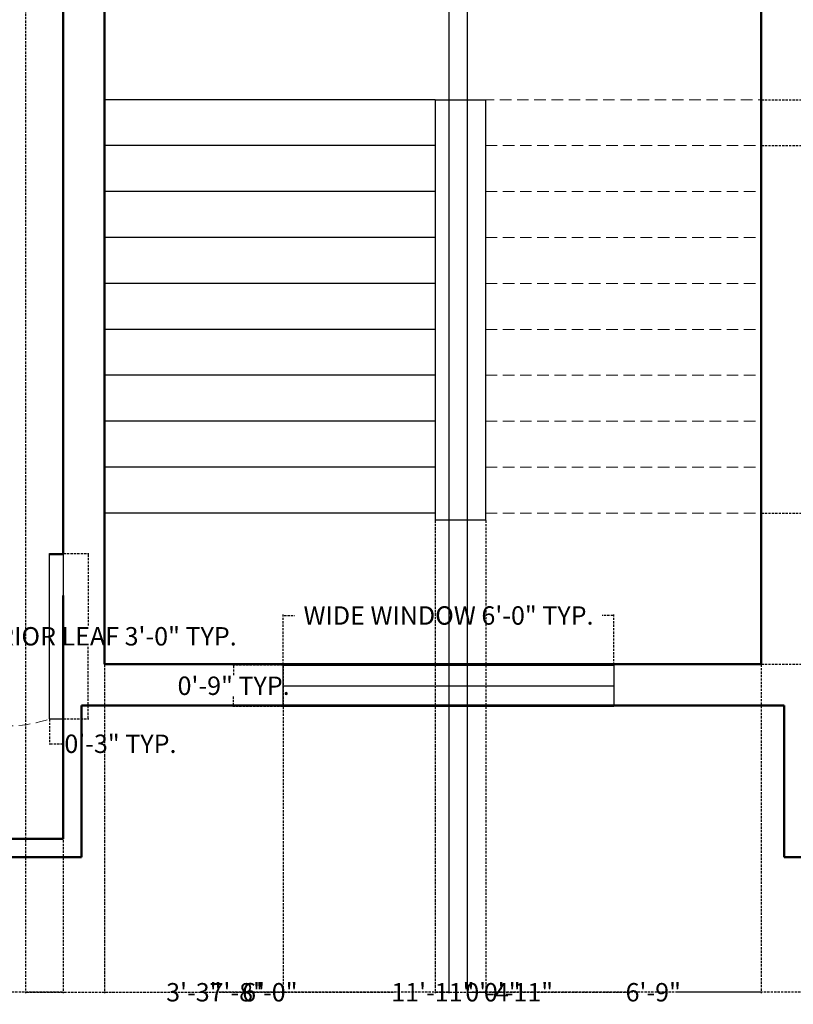
# Model space of a CAD drawing. Units: inches. Extents: x 513 to 1142, y 396 to 927.
# Tile 10 of 31: x 743 to 911, y 399 to 614. Entities that reach past the tile are written whole.
import ezdxf

# ---------------------------------------------------------------- set-up
doc = ezdxf.new("R2010")
doc.units = ezdxf.units.IN
doc.header["$MEASUREMENT"] = 0
doc.linetypes.add('DASHED', pattern=[0.75, 0.5, -0.25])
for name, color, linetype, lineweight in [('A-ANNO-DIMS', 2, 'DASHED', 18), ('A-DOOR', 4, 'Continuous', 25), ('A-DOOR-SWNG', 4, 'DASHED', 13), ('A-FLOR-STRS', 7, 'Continuous', 25), ('A-FLOR-STRS-OVHD', 7, 'DASHED', 18), ('A-WALL', 7, 'Continuous', 50), ('windows', 172, 'Continuous', 25)]:
    doc.layers.add(name, color=color, linetype=linetype, lineweight=lineweight)
doc.styles.get("Standard").update_dxf_attribs({"font": 'arial.ttf'})
doc.dimstyles.get("Standard").update_dxf_attribs({"dimtxt": 4, "dimasz": 0.18, "dimexe": 0.18, "dimexo": 0.0625, "dimgap": 0.09, "dimtad": 0, "dimtih": 1, "dimtoh": 1, "dimdec": 0, "dimrnd": 6, "dimzin": 0, "dimdsep": 46, "dimlunit": 3, "dimtxsty": 'Standard', "dimcen": 0.09, "dimadec": 0, "dimazin": 0, "dimtfac": 1, "dimtdec": 0, "dimtofl": 0, "dimtmove": 0, "dimatfit": 3, "dimfxl": 1, "dimtolj": 1, "dimtzin": 0, "dimarcsym": 0})

# ---------------------------------------------------------------- blocks, each defined once
blk = doc.blocks.new('WIN-72IN')
blk.add_line((0, 4.45), (72, 4.45))
blk.add_lwpolyline([(72, 9), (72, 0), (0, 0), (0, 9)], close=True)
blk = doc.blocks.new('DOOR-LEAF-36IN')
for p, q in [((0, 0), (0, 36)), ((0, 36), (3, 36)), ((3, 36), (3, 0)), ((0, 0), (3, 0))]:
    blk.add_line(p, q)
blk = doc.blocks.new('*D125')
at = {"layer": 'A-ANNO-DIMS', "color": 0, "lineweight": -2, "transparency": 16777216}
for p, q in [((752.06, 497.26), (757.58, 497.26)), ((757.4, 497.08), (757.4, 481.42)), ((757.4, 461.44), (757.4, 477.1)), ((752.06, 461.26), (757.58, 461.26))]:
    blk.add_line(p, q, dxfattribs=at)
at = {"layer": 'A-ANNO-DIMS', "color": 0, "transparency": 16777216}
for points in [[(757.37, 497.08), (757.43, 497.08), (757.4, 497.26)], [(757.37, 461.44), (757.43, 461.44), (757.4, 461.26)]]:
    blk.add_solid(points, dxfattribs=at)
at = {"layer": 'Defpoints', "color": 0, "transparency": 16777216}
for p in [(752, 497.26), (757.4, 497.26), (752, 461.26)]:
    blk.add_point(p, dxfattribs=at)
at = {"layer": 'A-ANNO-DIMS', "color": 0, "transparency": 16777216, "insert": (757.4, 479.26), "char_height": 4, "attachment_point": 5}
blk.add_mtext('\\A1;EXTERIOR LEAF 3\'-0" TYP.', dxfattribs=at)
blk = doc.blocks.new('*D126')
at = {"layer": 'A-ANNO-DIMS', "color": 0, "lineweight": -2, "transparency": 16777216}
for p, q in [((749, 461.2), (749, 455.68)), ((752, 461.2), (752, 455.68)), ((749.18, 455.86), (751.82, 455.86)), ((752, 455.86), (752.18, 455.86))]:
    blk.add_line(p, q, dxfattribs=at)
at = {"layer": 'A-ANNO-DIMS', "color": 0, "transparency": 16777216}
for points in [[(749.18, 455.89), (749.18, 455.83), (749, 455.86)], [(751.82, 455.89), (751.82, 455.83), (752, 455.86)]]:
    blk.add_solid(points, dxfattribs=at)
at = {"layer": 'Defpoints', "color": 0, "transparency": 16777216}
for p in [(749, 461.26), (752, 461.26), (752, 455.86)]:
    blk.add_point(p, dxfattribs=at)
at = {"layer": 'A-ANNO-DIMS', "color": 0, "transparency": 16777216, "insert": (764.46, 455.86), "char_height": 4, "attachment_point": 5}
blk.add_mtext('\\A1;0\'-3" TYP.', dxfattribs=at)
blk = doc.blocks.new('*D127')
at = {"layer": 'A-ANNO-DIMS', "color": 0, "lineweight": -2, "transparency": 16777216}
for p, q in [((799.91, 473.06), (799.91, 483.97)), ((800.09, 483.79), (802.44, 483.79)), ((871.73, 483.79), (869.38, 483.79)), ((871.91, 473.06), (871.91, 483.97))]:
    blk.add_line(p, q, dxfattribs=at)
at = {"layer": 'A-ANNO-DIMS', "color": 0, "transparency": 16777216}
for points in [[(800.09, 483.82), (800.09, 483.76), (799.91, 483.79)], [(871.73, 483.82), (871.73, 483.76), (871.91, 483.79)]]:
    blk.add_solid(points, dxfattribs=at)
at = {"layer": 'Defpoints', "color": 0, "transparency": 16777216}
for p in [(871.91, 483.79), (799.91, 472.99), (871.91, 472.99)]:
    blk.add_point(p, dxfattribs=at)
at = {"layer": 'A-ANNO-DIMS', "color": 0, "transparency": 16777216, "insert": (835.91, 483.79), "char_height": 4, "attachment_point": 5}
blk.add_mtext('\\A1;WIDE WINDOW 6\'-0" TYP.', dxfattribs=at)
blk = doc.blocks.new('*D128')
at = {"layer": 'A-ANNO-DIMS', "color": 0, "lineweight": -2, "transparency": 16777216}
for p, q in [((799.85, 472.99), (788.93, 472.99)), ((789.11, 472.81), (789.11, 470.63)), ((789.11, 464.17), (789.11, 466.36)), ((799.85, 463.99), (788.93, 463.99))]:
    blk.add_line(p, q, dxfattribs=at)
at = {"layer": 'A-ANNO-DIMS', "color": 0, "transparency": 16777216}
for points in [[(789.08, 472.81), (789.14, 472.81), (789.11, 472.99)], [(789.08, 464.17), (789.14, 464.17), (789.11, 463.99)]]:
    blk.add_solid(points, dxfattribs=at)
at = {"layer": 'Defpoints', "color": 0, "transparency": 16777216}
for p in [(789.11, 472.99), (799.91, 472.99), (799.91, 463.99)]:
    blk.add_point(p, dxfattribs=at)
at = {"layer": 'A-ANNO-DIMS', "color": 0, "transparency": 16777216, "insert": (789.11, 468.49), "char_height": 4, "attachment_point": 5}
blk.add_mtext('\\A1;0\'-9" TYP.', dxfattribs=at)
blk = doc.blocks.new('*D136')
at = {"layer": 'A-ANNO-DIMS', "color": 0, "lineweight": -2, "transparency": 16777216}
for p, q in [((836, 770.1), (836, 401.58)), ((743.8, 768.61), (743.8, 401.58)), ((743.98, 401.76), (784.51, 401.76)), ((835.82, 401.76), (795.29, 401.76))]:
    blk.add_line(p, q, dxfattribs=at)
at = {"layer": 'A-ANNO-DIMS', "color": 0, "transparency": 16777216}
for points in [[(743.98, 401.79), (743.98, 401.73), (743.8, 401.76)], [(835.82, 401.79), (835.82, 401.73), (836, 401.76)]]:
    blk.add_solid(points, dxfattribs=at)
at = {"layer": 'Defpoints', "color": 0, "transparency": 16777216}
for p in [(836, 770.16), (743.8, 768.67), (836, 401.76)]:
    blk.add_point(p, dxfattribs=at)
at = {"layer": 'A-ANNO-DIMS', "color": 0, "transparency": 16777216, "insert": (789.9, 401.76), "char_height": 4, "attachment_point": 5}
blk.add_mtext('\\A1;7\'-8"', dxfattribs=at)
blk = doc.blocks.new('*D137')
at = {"layer": 'A-ANNO-DIMS', "color": 0, "lineweight": -2, "transparency": 16777216}
for p, q in [((840, 770.1), (840, 401.58)), ((921, 770.07), (921, 401.58)), ((840.18, 401.76), (875.08, 401.76)), ((920.82, 401.76), (885.91, 401.76))]:
    blk.add_line(p, q, dxfattribs=at)
at = {"layer": 'A-ANNO-DIMS', "color": 0, "transparency": 16777216}
for points in [[(840.18, 401.79), (840.18, 401.73), (840, 401.76)], [(920.82, 401.79), (920.82, 401.73), (921, 401.76)]]:
    blk.add_solid(points, dxfattribs=at)
at = {"layer": 'Defpoints', "color": 0, "transparency": 16777216}
for p in [(840, 770.16), (921, 770.13), (921, 401.76)]:
    blk.add_point(p, dxfattribs=at)
at = {"layer": 'A-ANNO-DIMS', "color": 0, "transparency": 16777216, "insert": (880.5, 401.76), "char_height": 4, "attachment_point": 5}
blk.add_mtext('\\A1;6\'-9"', dxfattribs=at)
blk = doc.blocks.new('*D144')
at = {"layer": 'A-ANNO-DIMS', "color": 0, "lineweight": -2, "transparency": 16777216}
for p, q in [((584, 497.1), (584, 401.58)), ((752, 497.1), (752, 401.58)), ((584.18, 401.76), (661.22, 401.76)), ((751.82, 401.76), (674.77, 401.76))]:
    blk.add_line(p, q, dxfattribs=at)
at = {"layer": 'A-ANNO-DIMS', "color": 0, "transparency": 16777216}
for points in [[(584.18, 401.79), (584.18, 401.73), (584, 401.76)], [(751.82, 401.79), (751.82, 401.73), (752, 401.76)]]:
    blk.add_solid(points, dxfattribs=at)
at = {"layer": 'Defpoints', "color": 0, "transparency": 16777216}
for p in [(584, 497.16), (752, 497.16), (752, 401.76)]:
    blk.add_point(p, dxfattribs=at)
at = {"layer": 'A-ANNO-DIMS', "color": 0, "transparency": 16777216, "insert": (668, 401.76), "char_height": 4, "attachment_point": 5}
blk.add_mtext('\\A1;14\'-0"', dxfattribs=at)
blk = doc.blocks.new('*D145')
at = {"layer": 'A-ANNO-DIMS', "color": 0, "lineweight": -2, "transparency": 16777216}
for p, q in [((761, 473.1), (761, 401.58)), ((904, 473.1), (904, 401.58)), ((761.18, 401.76), (824.17, 401.76)), ((903.82, 401.76), (840.82, 401.76))]:
    blk.add_line(p, q, dxfattribs=at)
at = {"layer": 'A-ANNO-DIMS', "color": 0, "transparency": 16777216}
for points in [[(761.18, 401.79), (761.18, 401.73), (761, 401.76)], [(903.82, 401.79), (903.82, 401.73), (904, 401.76)]]:
    blk.add_solid(points, dxfattribs=at)
at = {"layer": 'Defpoints', "color": 0, "transparency": 16777216}
for p in [(761, 473.16), (904, 473.16), (904, 401.76)]:
    blk.add_point(p, dxfattribs=at)
at = {"layer": 'A-ANNO-DIMS', "color": 0, "transparency": 16777216, "insert": (832.5, 401.76), "char_height": 4, "attachment_point": 5}
blk.add_mtext('\\A1;11\'-11"', dxfattribs=at)
blk = doc.blocks.new('*D150')
at = {"layer": 'A-ANNO-DIMS', "color": 0, "lineweight": -2, "transparency": 16777216}
for p, q in [((904.06, 596.09), (1131.58, 596.09)), ((1131.4, 595.91), (1131.4, 553.23)), ((1131.4, 506.27), (1131.4, 548.96)), ((904.06, 506.09), (1131.58, 506.09))]:
    blk.add_line(p, q, dxfattribs=at)
at = {"layer": 'A-ANNO-DIMS', "color": 0, "transparency": 16777216}
for points in [[(1131.37, 595.91), (1131.43, 595.91), (1131.4, 596.09)], [(1131.37, 506.27), (1131.43, 506.27), (1131.4, 506.09)]]:
    blk.add_solid(points, dxfattribs=at)
at = {"layer": 'Defpoints', "color": 0, "transparency": 16777216}
for p in [(904, 596.09), (904, 506.09), (1131.4, 506.09)]:
    blk.add_point(p, dxfattribs=at)
at = {"layer": 'A-ANNO-DIMS', "color": 0, "transparency": 16777216, "insert": (1131.4, 551.09), "char_height": 4, "attachment_point": 5}
blk.add_mtext('\\A1;7\'-6"', dxfattribs=at)
blk = doc.blocks.new('*D151')
at = {"layer": 'A-ANNO-DIMS', "color": 0, "lineweight": -2, "transparency": 16777216}
for p, q in [((761, 506.03), (761, 401.58)), ((833, 506.03), (833, 401.58)), ((761.18, 401.76), (791.58, 401.76)), ((832.82, 401.76), (802.41, 401.76))]:
    blk.add_line(p, q, dxfattribs=at)
at = {"layer": 'A-ANNO-DIMS', "color": 0, "transparency": 16777216}
for points in [[(761.18, 401.79), (761.18, 401.73), (761, 401.76)], [(832.82, 401.79), (832.82, 401.73), (833, 401.76)]]:
    blk.add_solid(points, dxfattribs=at)
at = {"layer": 'Defpoints', "color": 0, "transparency": 16777216}
for p in [(761, 506.09), (833, 506.09), (833, 401.76)]:
    blk.add_point(p, dxfattribs=at)
at = {"layer": 'A-ANNO-DIMS', "color": 0, "transparency": 16777216, "insert": (797, 401.76), "char_height": 4, "attachment_point": 5}
blk.add_mtext('\\A1;6\'-0"', dxfattribs=at)
blk = doc.blocks.new('*D157')
at = {"layer": 'A-ANNO-DIMS', "color": 0, "lineweight": -2, "transparency": 16777216}
for p, q in [((761, 473.1), (761, 401.58)), ((799.91, 472.93), (799.91, 401.58)), ((761.18, 401.76), (775.05, 401.76)), ((799.73, 401.76), (785.86, 401.76))]:
    blk.add_line(p, q, dxfattribs=at)
at = {"layer": 'A-ANNO-DIMS', "color": 0, "transparency": 16777216}
for points in [[(761.18, 401.79), (761.18, 401.73), (761, 401.76)], [(799.73, 401.79), (799.73, 401.73), (799.91, 401.76)]]:
    blk.add_solid(points, dxfattribs=at)
at = {"layer": 'Defpoints', "color": 0, "transparency": 16777216}
for p in [(761, 473.16), (799.91, 472.99), (799.91, 401.76)]:
    blk.add_point(p, dxfattribs=at)
at = {"layer": 'A-ANNO-DIMS', "color": 0, "transparency": 16777216, "insert": (780.45, 401.76), "char_height": 4, "attachment_point": 5}
blk.add_mtext('\\A1;3\'-3"', dxfattribs=at)
blk = doc.blocks.new('*D169')
at = {"layer": 'A-ANNO-DIMS', "color": 0, "lineweight": -2, "transparency": 16777216}
for p, q in [((836, 774.1), (836, 401.58)), ((840, 774.1), (840, 401.58)), ((836.18, 401.76), (839.82, 401.76)), ((840, 401.76), (840.18, 401.76))]:
    blk.add_line(p, q, dxfattribs=at)
at = {"layer": 'A-ANNO-DIMS', "color": 0, "transparency": 16777216}
for points in [[(836.18, 401.79), (836.18, 401.73), (836, 401.76)], [(839.82, 401.79), (839.82, 401.73), (840, 401.76)]]:
    blk.add_solid(points, dxfattribs=at)
at = {"layer": 'Defpoints', "color": 0, "transparency": 16777216}
for p in [(836, 774.16), (840, 774.16), (840, 401.76)]:
    blk.add_point(p, dxfattribs=at)
at = {"layer": 'A-ANNO-DIMS', "color": 0, "transparency": 16777216, "insert": (845.58, 401.76), "char_height": 4, "attachment_point": 5}
blk.add_mtext('\\A1;0\'-4"', dxfattribs=at)
blk = doc.blocks.new('*D171')
at = {"layer": 'A-ANNO-DIMS', "color": 0, "lineweight": -2, "transparency": 16777216}
for p, q in [((904.06, 596.09), (1131.58, 596.09)), ((1131.4, 595.91), (1131.4, 593.23)), ((1131.4, 586.27), (1131.4, 588.96)), ((904.06, 586.09), (1131.58, 586.09))]:
    blk.add_line(p, q, dxfattribs=at)
at = {"layer": 'A-ANNO-DIMS', "color": 0, "transparency": 16777216}
for points in [[(1131.37, 595.91), (1131.43, 595.91), (1131.4, 596.09)], [(1131.37, 586.27), (1131.43, 586.27), (1131.4, 586.09)]]:
    blk.add_solid(points, dxfattribs=at)
at = {"layer": 'Defpoints', "color": 0, "transparency": 16777216}
for p in [(904, 596.09), (904, 586.09), (1131.4, 586.09)]:
    blk.add_point(p, dxfattribs=at)
at = {"layer": 'A-ANNO-DIMS', "color": 0, "transparency": 16777216, "insert": (1131.4, 591.09), "char_height": 4, "attachment_point": 5}
blk.add_mtext('\\A1;0\'-10"', dxfattribs=at)
blk = doc.blocks.new('*D172')
at = {"layer": 'A-ANNO-DIMS', "color": 0, "lineweight": -2, "transparency": 16777216}
for p, q in [((904.06, 506.09), (1131.58, 506.09)), ((1131.4, 505.91), (1131.4, 491.76)), ((1131.4, 473.34), (1131.4, 487.49)), ((904.06, 473.16), (1131.58, 473.16))]:
    blk.add_line(p, q, dxfattribs=at)
at = {"layer": 'A-ANNO-DIMS', "color": 0, "transparency": 16777216}
for points in [[(1131.37, 505.91), (1131.43, 505.91), (1131.4, 506.09)], [(1131.37, 473.34), (1131.43, 473.34), (1131.4, 473.16)]]:
    blk.add_solid(points, dxfattribs=at)
at = {"layer": 'Defpoints', "color": 0, "transparency": 16777216}
for p in [(904, 506.09), (904, 473.16), (1131.4, 473.16)]:
    blk.add_point(p, dxfattribs=at)
at = {"layer": 'A-ANNO-DIMS', "color": 0, "transparency": 16777216, "insert": (1131.4, 489.63), "char_height": 4, "attachment_point": 5}
blk.add_mtext('\\A1;2\'-9"', dxfattribs=at)
blk = doc.blocks.new('*D173')
at = {"layer": 'A-ANNO-DIMS', "color": 0, "lineweight": -2, "transparency": 16777216}
for p, q in [((904.06, 637.16), (1131.58, 637.16)), ((1131.4, 636.98), (1131.4, 618.76)), ((1131.4, 596.27), (1131.4, 614.49)), ((904.06, 596.09), (1131.58, 596.09))]:
    blk.add_line(p, q, dxfattribs=at)
at = {"layer": 'A-ANNO-DIMS', "color": 0, "transparency": 16777216}
for points in [[(1131.37, 636.98), (1131.43, 636.98), (1131.4, 637.16)], [(1131.37, 596.27), (1131.43, 596.27), (1131.4, 596.09)]]:
    blk.add_solid(points, dxfattribs=at)
at = {"layer": 'Defpoints', "color": 0, "transparency": 16777216}
for p in [(904, 637.16), (1131.4, 637.16), (904, 596.09)]:
    blk.add_point(p, dxfattribs=at)
at = {"layer": 'A-ANNO-DIMS', "color": 0, "transparency": 16777216, "insert": (1131.4, 616.63), "char_height": 4, "attachment_point": 5}
blk.add_mtext('\\A1;3\'-5"', dxfattribs=at)
blk = doc.blocks.new('*D174')
at = {"layer": 'A-ANNO-DIMS', "color": 0, "lineweight": -2, "transparency": 16777216}
for p, q in [((833, 504.46), (833, 401.58)), ((844, 504.46), (844, 401.58)), ((833.18, 401.76), (843.82, 401.76)), ((844, 401.76), (844.18, 401.76))]:
    blk.add_line(p, q, dxfattribs=at)
at = {"layer": 'A-ANNO-DIMS', "color": 0, "transparency": 16777216}
for points in [[(833.18, 401.79), (833.18, 401.73), (833, 401.76)], [(843.82, 401.79), (843.82, 401.73), (844, 401.76)]]:
    blk.add_solid(points, dxfattribs=at)
at = {"layer": 'Defpoints', "color": 0, "transparency": 16777216}
for p in [(833, 504.53), (844, 504.53), (844, 401.76)]:
    blk.add_point(p, dxfattribs=at)
at = {"layer": 'A-ANNO-DIMS', "color": 0, "transparency": 16777216, "insert": (851.14, 401.76), "char_height": 4, "attachment_point": 5}
blk.add_mtext('\\A1;0\'-11"', dxfattribs=at)

msp = doc.modelspace()

# ---------------------------------------------------------------- linework, layer by layer
at = {"layer": 'A-DOOR-SWNG', "ltscale": 5}
msp.add_arc((739.87, 488.11), 28.36, 161.3835, 288.7781, dxfattribs=at)
at = {"layer": 'A-FLOR-STRS'}
for p, q in [((833, 596.09), (761, 596.09)), ((833, 596.09), (833, 504.53)), ((833, 596.09), (844, 596.09)), ((844, 504.53), (844, 596.09)), ((833, 586.09), (761, 586.09)), ((833, 576.09), (761, 576.09)), ((833, 566.09), (761, 566.09)), ((833, 556.09), (761, 556.09)), ((833, 546.09), (761, 546.09)), ((833, 536.09), (761, 536.09)), ((833, 526.09), (761, 526.09)), ((833, 516.09), (761, 516.09)), ((833, 506.09), (761, 506.09)), ((844, 504.53), (833, 504.53))]:
    msp.add_line(p, q, dxfattribs=at)
at = {"layer": 'A-FLOR-STRS-OVHD', "ltscale": 5}
for p, q in [((843.34, 596.09), (904, 596.09)), ((844, 586.09), (904, 586.09)), ((844, 576.09), (904, 576.09)), ((844, 566.09), (904, 566.09)), ((844, 556.09), (904, 556.09)), ((844, 546.09), (904, 546.09)), ((844, 536.09), (904, 536.09)), ((844, 526.09), (904, 526.09)), ((844, 516.09), (904, 516.09)), ((844, 506.09), (904, 506.09))]:
    msp.add_line(p, q, dxfattribs=at)
at = {"layer": 'A-WALL'}
for p, q in [((752, 641.16), (752, 497.16)), ((761, 637.16), (761, 473.16)), ((904, 473.16), (904, 637.16)), ((749, 497.16), (752, 497.16)), ((752, 488.16), (752, 435.16)), ((761, 473.16), (904, 473.16)), ((756, 464.16), (909, 464.16)), ((756, 464.16), (756, 431.16)), ((909, 431.16), (909, 464.16)), ((579, 435.16), (752, 435.16)), ((575, 431.16), (756, 431.16)), ((909, 431.16), (1090, 431.16))]:
    msp.add_line(p, q, dxfattribs=at)

# ---------------------------------------------------------------- block references
at = {"layer": 'A-DOOR'}
msp.add_blockref('DOOR-LEAF-36IN', (749, 461.26), dxfattribs=at)
at = {"layer": 'windows'}
msp.add_blockref('WIN-72IN', (799.91, 463.99), dxfattribs=at)

# ---------------------------------------------------------------- dimensions: what is measured, and where the dimension line sits
at = {"layer": 'A-ANNO-DIMS'}
for base, p1, p2, picture, middle in [((840, 401.76), (836, 774.16), (840, 774.16), '*D169', (845.58, 401.76)), ((836, 401.76), (743.8, 768.67), (836, 770.16), '*D136', (789.9, 401.76)), ((921, 401.76), (840, 770.16), (921, 770.13), '*D137', (880.5, 401.76)), ((833, 401.76), (761, 506.09), (833, 506.09), '*D151', (797, 401.76)), ((844, 401.76), (833, 504.53), (844, 504.53), '*D174', (851.14, 401.76)), ((752, 401.76), (584, 497.16), (752, 497.16), '*D144', (668, 401.76)), ((904, 401.76), (761, 473.16), (904, 473.16), '*D145', (832.5, 401.76)), ((799.91, 401.76), (761, 473.16), (799.91, 472.99), '*D157', (780.45, 401.76))]:
    dim = msp.add_linear_dim(base=base, p1=p1, p2=p2, dimstyle='Standard', override={"dimdec": 1, "dimlfac": 1, "dimrnd": 0, "dimzin": 1, "dimdsep": 46, "dimlunit": 4, "dimfrac": 2}, dxfattribs=at)
    dim.commit()
    dim.dimension.update_dxf_attribs({"geometry": picture, "text_midpoint": middle})
for base, p1, p2, picture, middle in [((1131.4, 637.16), (904, 596.09), (904, 637.16), '*D173', (1131.4, 616.63)), ((1131.4, 506.09), (904, 596.09), (904, 506.09), '*D150', (1131.4, 551.09)), ((1131.4, 586.09), (904, 596.09), (904, 586.09), '*D171', (1131.4, 591.09)), ((1131.4, 473.16), (904, 506.09), (904, 473.16), '*D172', (1131.4, 489.63))]:
    dim = msp.add_linear_dim(base=base, p1=p1, p2=p2, angle=90, dimstyle='Standard', override={"dimdec": 1, "dimlfac": 1, "dimrnd": 0, "dimzin": 1, "dimdsep": 46, "dimlunit": 4, "dimfrac": 2}, dxfattribs=at)
    dim.commit()
    dim.dimension.update_dxf_attribs({"geometry": picture, "text_midpoint": middle})
for base, p1, p2, text, picture, middle in [((757.4, 497.26), (752, 461.26), (752, 497.26), 'EXTERIOR LEAF <> TYP.', '*D125', (757.4, 479.26)), ((789.11, 472.99), (799.91, 463.99), (799.91, 472.99), '<> TYP.', '*D128', (789.11, 468.49))]:
    dim = msp.add_linear_dim(base=base, p1=p1, p2=p2, angle=90, text=text, dimstyle='Standard', override={"dimdec": 1, "dimlfac": 1, "dimrnd": 0, "dimzin": 1, "dimdsep": 46, "dimlunit": 4, "dimfrac": 2}, dxfattribs=at)
    dim.commit()
    dim.dimension.update_dxf_attribs({"geometry": picture, "text_midpoint": middle})
for base, p1, p2, text, picture, middle in [((871.91, 483.79), (799.91, 472.99), (871.91, 472.99), 'WIDE WINDOW <> TYP.', '*D127', (835.91, 483.79)), ((752, 455.86), (749, 461.26), (752, 461.26), '<> TYP.', '*D126', (764.46, 455.86))]:
    dim = msp.add_linear_dim(base=base, p1=p1, p2=p2, text=text, dimstyle='Standard', override={"dimdec": 1, "dimlfac": 1, "dimrnd": 0, "dimzin": 1, "dimdsep": 46, "dimlunit": 4, "dimfrac": 2}, dxfattribs=at)
    dim.commit()
    dim.dimension.update_dxf_attribs({"geometry": picture, "text_midpoint": middle})

doc.saveas('drawing.dxf')
